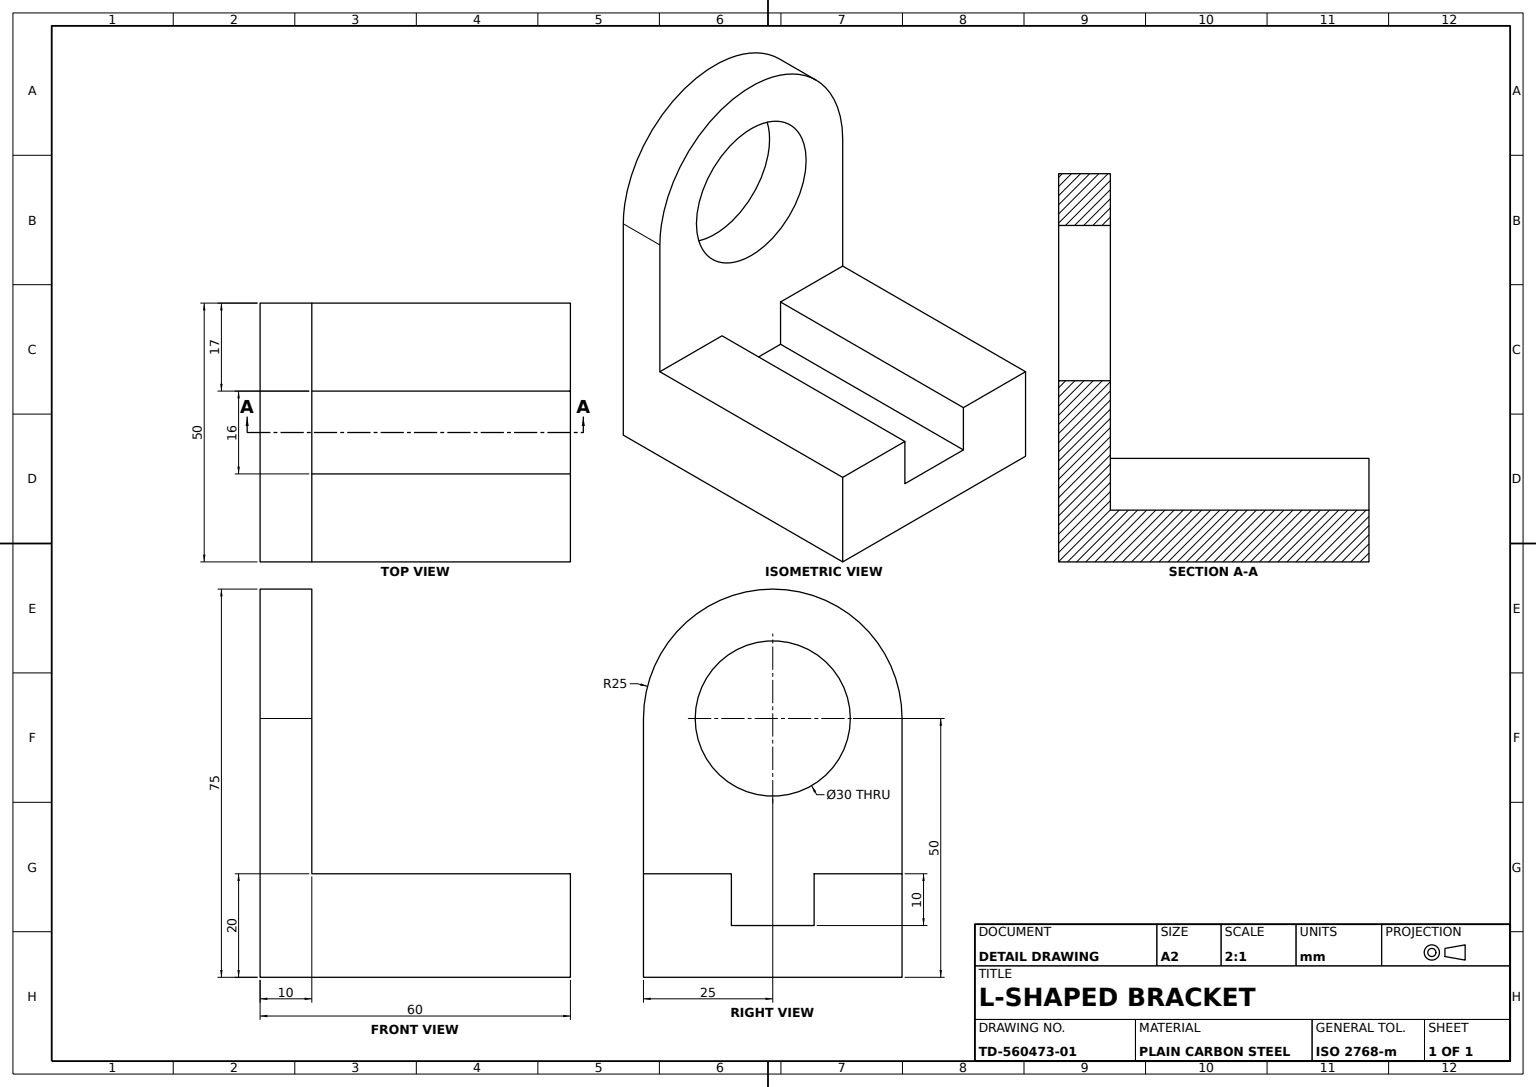
SolidWorks part; units mm, degrees
material "Plain Carbon Steel"
ref_plane "Front Plane" through (0, 0, 0) normal (0, 0, 1) x (1, 0, 0)
ref_plane "Top Plane" through (0, 0, 0) normal (0, 1, 0) x (1, 0, 0)
ref_plane "Right Plane" through (0, 0, 0) normal (1, 0, 0) x (0, 0, -1)
sketch "Base Block Sketch" plane through (0, 0, 0) normal (0, 1, 0) x (1, 0, 0)
  line L1 (-30, 25) -> (30, 25)
  line L2 (-30, 25) -> (-30, -25)
  line L3 (-30, -25) -> (30, -25)
  line L4 (30, 25) -> (30, -25)
  line L5 (-30, 25) -> (30, -25) construction
  line L6 (-30, -25) -> (30, 25) construction
  point P0 (0, 0)
  dimension "D1" = 50
  dimension "D2" = 60
extrude "Base Block" add sketch "Base Block Sketch" along normal blind 20
sketch "Upright Sketch" plane through (0, 20, 0) normal (0, 1, 0) x (1, 0, 0)
  line L0 (-30, 25) -> (-20, 25)
  line L1 (30, 25) -> (-30, 25) construction
  line L2 (-20, 25) -> (-20, -25)
  line L3 (-30, -25) -> (30, -25) construction
  line L4 (-20, -25) -> (-30, -25)
  line L5 (-30, 25) -> (-30, -25) construction
  line L6 (-30, -25) -> (-30, 25)
  dimension "D1" = 10
extrude "Upright" add sketch "Upright Sketch" along normal blind 30
sketch "Rounded Top Sketch" plane through (-20, 0, 0) normal (1, 0, 0) x (0, 0, -1)
  line L0 (-25, 50) -> (25, 50) construction
  circle A0 centre (0, 50) radius 25
extrude "Rounded Top" add sketch "Rounded Top Sketch" against normal blind 10
sketch "Pivot Hole Sketch" plane through (-20, 0, 0) normal (1, 0, 0) x (0, 0, -1)
  circle A0 centre (0, 50) radius 15
  dimension "D1" = 30
extrude "Pivot Hole" cut sketch "Pivot Hole Sketch" against normal blind 10
sketch "Base Slot Sketch" plane through (30, 0, 0) normal (1, 0, 0) x (0, 0, -1)
  line L0 (-8, 20) -> (-8, 10)
  line L1 (-25, 20) -> (25, 20) construction
  line L2 (-8, 10) -> (8, 10)
  line L3 (8, 10) -> (8, 20)
  line L4 (8, 20) -> (-8, 20)
  line L5 (-25, 20) -> (-25, 0) construction
  line L6 (25, 20) -> (25, 0) construction
  dimension "D1" = 17
  dimension "D2" = 17
  dimension "D3" = 10
extrude "Base Slot" cut sketch "Base Slot Sketch" against normal blind 50
